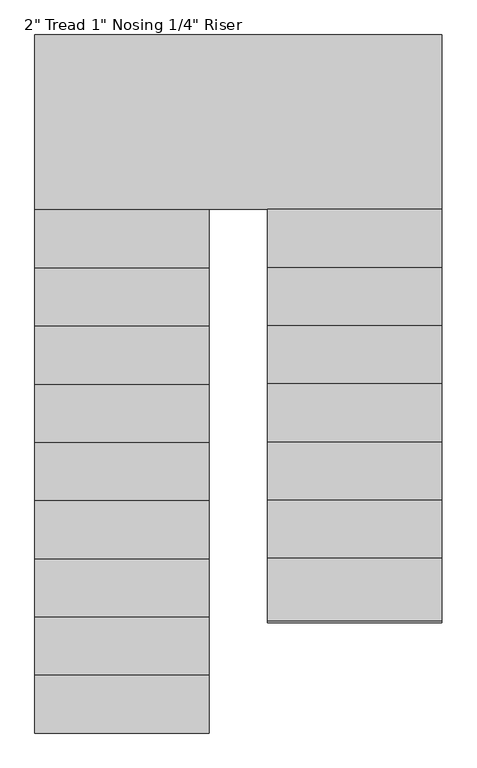
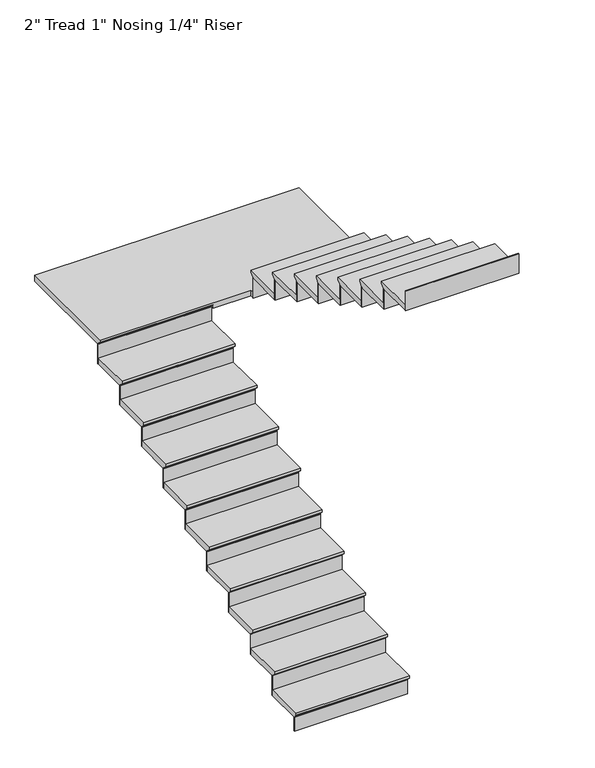
"""IFC4 building model written with IfcOpenShell, lengths in millimetres: stair flight geometry."""

from ifc_helpers import new_model, si_unit, origin, place, context, project, spatial, faceted_brep, source, transform, mapped, element, save


def stair_flight_5b78524c(model_context):
    return source(origin(), model_context, "Body", "Brep", [
        faceted_brep([(-77.7175798, -12221.8061634, 455.0833333), (-77.7175798, -12221.8061634, 474.1333333), (-992.1175798, -12221.8061634, 474.1333333), (-992.1175798, -12221.8061634, 455.0833333), (-77.7175798, -12196.4061634, 429.6833333), (-992.1175798, -12196.4061634, 429.6833333), (-77.7175798, -11891.6061634, 474.1333333), (-992.1175798, -11891.6061634, 474.1333333), (-992.1175798, -12196.4061634, 423.3333333), (-992.1175798, -11891.6061634, 423.3333333), (-77.7175798, -11891.6061634, 423.3333333), (-77.7175798, -12196.4061634, 423.3333333)], [[[0, 1, 2, 3]], [[4, 0, 3, 5]], [[2, 1, 6, 7]], [[8, 9, 10, 11]], [[2, 7, 9, 8, 5, 3]], [[8, 11, 4, 5]], [[6, 1, 0, 4, 11, 10]], [[7, 6, 10, 9]]]),
        faceted_brep([(-77.7175798, -12196.4061634, 423.3333333), (-77.7175798, -12196.4061634, 304.8), (-77.7175798, -12190.0561634, 304.8), (-77.7175798, -12190.0561634, 423.3333333), (-992.1175798, -12196.4061634, 423.3333333), (-992.1175798, -12190.0561634, 423.3333333), (-992.1175798, -12190.0561634, 304.8), (-992.1175798, -12196.4061634, 304.8)], [[[0, 1, 2, 3]], [[4, 5, 6, 7]], [[1, 0, 4, 7]], [[2, 1, 7, 6]], [[3, 2, 6, 5]], [[0, 3, 5, 4]]]),
        faceted_brep([(-77.7175798, -11891.6061634, 592.6666667), (-77.7175798, -11891.6061634, 423.3333333), (-77.7175798, -11885.2561634, 423.3333333), (-77.7175798, -11885.2561634, 592.6666667), (-992.1175798, -11891.6061634, 592.6666667), (-992.1175798, -11885.2561634, 592.6666667), (-992.1175798, -11885.2561634, 423.3333333), (-992.1175798, -11891.6061634, 423.3333333)], [[[0, 1, 2, 3]], [[4, 5, 6, 7]], [[1, 0, 4, 7]], [[2, 1, 7, 6]], [[3, 2, 6, 5]], [[0, 3, 5, 4]]]),
        faceted_brep([(-992.1175798, -11917.0061634, 643.4666667), (-77.7175798, -11917.0061634, 643.4666667), (-77.7175798, -11586.8061634, 643.4666667), (-992.1175798, -11586.8061634, 643.4666667), (-992.1175798, -11891.6061634, 592.6666667), (-992.1175798, -11586.8061634, 592.6666667), (-77.7175798, -11586.8061634, 592.6666667), (-77.7175798, -11891.6061634, 592.6666667), (-992.1175798, -11891.6061634, 599.0166667), (-992.1175798, -11917.0061634, 624.4166667), (-77.7175798, -11891.6061634, 599.0166667), (-77.7175798, -11917.0061634, 624.4166667)], [[[0, 1, 2, 3]], [[4, 5, 6, 7]], [[0, 3, 5, 4, 8, 9]], [[4, 7, 10, 8]], [[2, 1, 11, 10, 7, 6]], [[3, 2, 6, 5]], [[11, 1, 0, 9]], [[10, 11, 9, 8]]]),
        faceted_brep([(-77.7175798, -11586.8061634, 762.0), (-77.7175798, -11586.8061634, 592.6666667), (-77.7175798, -11580.4561634, 592.6666667), (-77.7175798, -11580.4561634, 762.0), (-992.1175798, -11586.8061634, 762.0), (-992.1175798, -11580.4561634, 762.0), (-992.1175798, -11580.4561634, 592.6666667), (-992.1175798, -11586.8061634, 592.6666667)], [[[0, 1, 2, 3]], [[4, 5, 6, 7]], [[1, 0, 4, 7]], [[2, 1, 7, 6]], [[3, 2, 6, 5]], [[0, 3, 5, 4]]]),
        faceted_brep([(-992.1175798, -11612.2061634, 812.8), (-77.7175798, -11612.2061634, 812.8), (-77.7175798, -11282.0061634, 812.8), (-992.1175798, -11282.0061634, 812.8), (-992.1175798, -11586.8061634, 762.0), (-992.1175798, -11282.0061634, 762.0), (-77.7175798, -11282.0061634, 762.0), (-77.7175798, -11586.8061634, 762.0), (-992.1175798, -11586.8061634, 768.35), (-992.1175798, -11612.2061634, 793.75), (-77.7175798, -11586.8061634, 768.35), (-77.7175798, -11612.2061634, 793.75)], [[[0, 1, 2, 3]], [[4, 5, 6, 7]], [[0, 3, 5, 4, 8, 9]], [[4, 7, 10, 8]], [[2, 1, 11, 10, 7, 6]], [[3, 2, 6, 5]], [[11, 1, 0, 9]], [[10, 11, 9, 8]]]),
        faceted_brep([(-77.7175798, -11282.0061634, 931.3333333), (-77.7175798, -11282.0061634, 762.0), (-77.7175798, -11275.6561634, 762.0), (-77.7175798, -11275.6561634, 931.3333333), (-992.1175798, -11282.0061634, 931.3333333), (-992.1175798, -11275.6561634, 931.3333333), (-992.1175798, -11275.6561634, 762.0), (-992.1175798, -11282.0061634, 762.0)], [[[0, 1, 2, 3]], [[4, 5, 6, 7]], [[1, 0, 4, 7]], [[2, 1, 7, 6]], [[3, 2, 6, 5]], [[0, 3, 5, 4]]]),
        faceted_brep([(-992.1175798, -11307.4061634, 982.1333333), (-77.7175798, -11307.4061634, 982.1333333), (-77.7175798, -10977.2061634, 982.1333333), (-992.1175798, -10977.2061634, 982.1333333), (-992.1175798, -11282.0061634, 931.3333333), (-992.1175798, -10977.2061634, 931.3333333), (-77.7175798, -10977.2061634, 931.3333333), (-77.7175798, -11282.0061634, 931.3333333), (-992.1175798, -11282.0061634, 937.6833333), (-992.1175798, -11307.4061634, 963.0833333), (-77.7175798, -11282.0061634, 937.6833333), (-77.7175798, -11307.4061634, 963.0833333)], [[[0, 1, 2, 3]], [[4, 5, 6, 7]], [[0, 3, 5, 4, 8, 9]], [[4, 7, 10, 8]], [[2, 1, 11, 10, 7, 6]], [[3, 2, 6, 5]], [[11, 1, 0, 9]], [[10, 11, 9, 8]]]),
        faceted_brep([(-77.7175798, -10977.2061634, 1100.6666667), (-77.7175798, -10977.2061634, 931.3333333), (-77.7175798, -10970.8561634, 931.3333333), (-77.7175798, -10970.8561634, 1100.6666667), (-992.1175798, -10977.2061634, 1100.6666667), (-992.1175798, -10970.8561634, 1100.6666667), (-992.1175798, -10970.8561634, 931.3333333), (-992.1175798, -10977.2061634, 931.3333333)], [[[0, 1, 2, 3]], [[4, 5, 6, 7]], [[1, 0, 4, 7]], [[2, 1, 7, 6]], [[3, 2, 6, 5]], [[0, 3, 5, 4]]]),
        faceted_brep([(-992.1175798, -11002.6061634, 1151.4666667), (-77.7175798, -11002.6061634, 1151.4666667), (-77.7175798, -10672.4061634, 1151.4666667), (-992.1175798, -10672.4061634, 1151.4666667), (-992.1175798, -10977.2061634, 1100.6666667), (-992.1175798, -10672.4061634, 1100.6666667), (-77.7175798, -10672.4061634, 1100.6666667), (-77.7175798, -10977.2061634, 1100.6666667), (-992.1175798, -10977.2061634, 1107.0166667), (-992.1175798, -11002.6061634, 1132.4166667), (-77.7175798, -10977.2061634, 1107.0166667), (-77.7175798, -11002.6061634, 1132.4166667)], [[[0, 1, 2, 3]], [[4, 5, 6, 7]], [[0, 3, 5, 4, 8, 9]], [[4, 7, 10, 8]], [[2, 1, 11, 10, 7, 6]], [[3, 2, 6, 5]], [[11, 1, 0, 9]], [[10, 11, 9, 8]]]),
        faceted_brep([(-77.7175798, -10672.4061634, 1270.0), (-77.7175798, -10672.4061634, 1100.6666667), (-77.7175798, -10666.0561634, 1100.6666667), (-77.7175798, -10666.0561634, 1270.0), (-992.1175798, -10672.4061634, 1270.0), (-992.1175798, -10666.0561634, 1270.0), (-992.1175798, -10666.0561634, 1100.6666667), (-992.1175798, -10672.4061634, 1100.6666667)], [[[0, 1, 2, 3]], [[4, 5, 6, 7]], [[1, 0, 4, 7]], [[2, 1, 7, 6]], [[3, 2, 6, 5]], [[0, 3, 5, 4]]]),
        faceted_brep([(-992.1175798, -10697.8061634, 1320.8), (-77.7175798, -10697.8061634, 1320.8), (-77.7175798, -10367.6061634, 1320.8), (-992.1175798, -10367.6061634, 1320.8), (-992.1175798, -10672.4061634, 1270.0), (-992.1175798, -10367.6061634, 1270.0), (-77.7175798, -10367.6061634, 1270.0), (-77.7175798, -10672.4061634, 1270.0), (-992.1175798, -10672.4061634, 1276.35), (-992.1175798, -10697.8061634, 1301.75), (-77.7175798, -10672.4061634, 1276.35), (-77.7175798, -10697.8061634, 1301.75)], [[[0, 1, 2, 3]], [[4, 5, 6, 7]], [[0, 3, 5, 4, 8, 9]], [[4, 7, 10, 8]], [[2, 1, 11, 10, 7, 6]], [[3, 2, 6, 5]], [[11, 1, 0, 9]], [[10, 11, 9, 8]]]),
        faceted_brep([(-77.7175798, -10367.6061634, 1439.3333333), (-77.7175798, -10367.6061634, 1270.0), (-77.7175798, -10361.2561634, 1270.0), (-77.7175798, -10361.2561634, 1439.3333333), (-992.1175798, -10367.6061634, 1439.3333333), (-992.1175798, -10361.2561634, 1439.3333333), (-992.1175798, -10361.2561634, 1270.0), (-992.1175798, -10367.6061634, 1270.0)], [[[0, 1, 2, 3]], [[4, 5, 6, 7]], [[1, 0, 4, 7]], [[2, 1, 7, 6]], [[3, 2, 6, 5]], [[0, 3, 5, 4]]]),
        faceted_brep([(-992.1175798, -10393.0061634, 1490.1333333), (-77.7175798, -10393.0061634, 1490.1333333), (-77.7175798, -10062.8061634, 1490.1333333), (-992.1175798, -10062.8061634, 1490.1333333), (-992.1175798, -10367.6061634, 1439.3333333), (-992.1175798, -10062.8061634, 1439.3333333), (-77.7175798, -10062.8061634, 1439.3333333), (-77.7175798, -10367.6061634, 1439.3333333), (-992.1175798, -10367.6061634, 1445.6833333), (-992.1175798, -10393.0061634, 1471.0833333), (-77.7175798, -10367.6061634, 1445.6833333), (-77.7175798, -10393.0061634, 1471.0833333)], [[[0, 1, 2, 3]], [[4, 5, 6, 7]], [[0, 3, 5, 4, 8, 9]], [[4, 7, 10, 8]], [[2, 1, 11, 10, 7, 6]], [[3, 2, 6, 5]], [[11, 1, 0, 9]], [[10, 11, 9, 8]]]),
        faceted_brep([(-77.7175798, -10062.8061634, 1608.6666667), (-77.7175798, -10062.8061634, 1439.3333333), (-77.7175798, -10056.4561634, 1439.3333333), (-77.7175798, -10056.4561634, 1608.6666667), (-992.1175798, -10062.8061634, 1608.6666667), (-992.1175798, -10056.4561634, 1608.6666667), (-992.1175798, -10056.4561634, 1439.3333333), (-992.1175798, -10062.8061634, 1439.3333333)], [[[0, 1, 2, 3]], [[4, 5, 6, 7]], [[1, 0, 4, 7]], [[2, 1, 7, 6]], [[3, 2, 6, 5]], [[0, 3, 5, 4]]]),
        faceted_brep([(-992.1175798, -10088.2061634, 1659.4666667), (-77.7175798, -10088.2061634, 1659.4666667), (-77.7175798, -9758.0061634, 1659.4666667), (-992.1175798, -9758.0061634, 1659.4666667), (-992.1175798, -10062.8061634, 1608.6666667), (-992.1175798, -9758.0061634, 1608.6666667), (-77.7175798, -9758.0061634, 1608.6666667), (-77.7175798, -10062.8061634, 1608.6666667), (-992.1175798, -10062.8061634, 1615.0166667), (-992.1175798, -10088.2061634, 1640.4166667), (-77.7175798, -10062.8061634, 1615.0166667), (-77.7175798, -10088.2061634, 1640.4166667)], [[[0, 1, 2, 3]], [[4, 5, 6, 7]], [[0, 3, 5, 4, 8, 9]], [[4, 7, 10, 8]], [[2, 1, 11, 10, 7, 6]], [[3, 2, 6, 5]], [[11, 1, 0, 9]], [[10, 11, 9, 8]]]),
        faceted_brep([(-77.7175798, -9758.0061634, 1778.0), (-77.7175798, -9758.0061634, 1608.6666667), (-77.7175798, -9751.6561634, 1608.6666667), (-77.7175798, -9751.6561634, 1778.0), (-992.1175798, -9758.0061634, 1778.0), (-992.1175798, -9751.6561634, 1778.0), (-992.1175798, -9751.6561634, 1608.6666667), (-992.1175798, -9758.0061634, 1608.6666667)], [[[0, 1, 2, 3]], [[4, 5, 6, 7]], [[1, 0, 4, 7]], [[2, 1, 7, 6]], [[3, 2, 6, 5]], [[0, 3, 5, 4]]]),
        faceted_brep([(-992.1175798, -9783.4061634, 1828.8), (-77.7175798, -9783.4061634, 1828.8), (-77.7175798, -9453.2061634, 1828.8), (-992.1175798, -9453.2061634, 1828.8), (-992.1175798, -9758.0061634, 1778.0), (-992.1175798, -9453.2061634, 1778.0), (-77.7175798, -9453.2061634, 1778.0), (-77.7175798, -9758.0061634, 1778.0), (-992.1175798, -9758.0061634, 1784.35), (-992.1175798, -9783.4061634, 1809.75), (-77.7175798, -9758.0061634, 1784.35), (-77.7175798, -9783.4061634, 1809.75)], [[[0, 1, 2, 3]], [[4, 5, 6, 7]], [[0, 3, 5, 4, 8, 9]], [[4, 7, 10, 8]], [[2, 1, 11, 10, 7, 6]], [[3, 2, 6, 5]], [[11, 1, 0, 9]], [[10, 11, 9, 8]]]),
        faceted_brep([(-77.7175798, -9453.2061634, 1947.3333333), (-77.7175798, -9453.2061634, 1778.0), (-77.7175798, -9446.8561634, 1778.0), (-77.7175798, -9446.8561634, 1947.3333333), (-992.1175798, -9453.2061634, 1947.3333333), (-992.1175798, -9446.8561634, 1947.3333333), (-992.1175798, -9446.8561634, 1778.0), (-992.1175798, -9453.2061634, 1778.0)], [[[0, 1, 2, 3]], [[4, 5, 6, 7]], [[1, 0, 4, 7]], [[2, 1, 7, 6]], [[3, 2, 6, 5]], [[0, 3, 5, 4]]]),
        faceted_brep([(1141.4824202, -9504.0061634, 1998.1333333), (1141.4824202, -8564.2061634, 1998.1333333), (-992.1175798, -8564.2061634, 1998.1333333), (-992.1175798, -9478.6061634, 1998.1333333), (227.0824202, -9478.6061634, 1998.1333333), (227.0824202, -9504.0061634, 1998.1333333), (1141.4824202, -8564.2061634, 1947.3333333), (1141.4824202, -9504.0061634, 1947.3333333), (227.0824202, -9504.0061634, 1947.3333333), (227.0824202, -9478.6061634, 1947.3333333), (-77.7175798, -9478.6061634, 1947.3333333), (-77.7175798, -9453.2061634, 1947.3333333), (-992.1175798, -9453.2061634, 1947.3333333), (-992.1175798, -8564.2061634, 1947.3333333), (-992.1175798, -9453.2061634, 1953.6833333), (-992.1175798, -9478.6061634, 1979.0833333), (-77.7175798, -9453.2061634, 1953.6833333), (-77.7175798, -9478.6061634, 1979.0833333)], [[[0, 1, 2, 3, 4, 5]], [[6, 7, 8, 9, 10, 11, 12, 13]], [[1, 0, 7, 6]], [[2, 1, 6, 13]], [[3, 2, 13, 12, 14, 15]], [[12, 11, 16, 14]], [[11, 10, 17, 16]], [[4, 3, 15, 17, 10, 9]], [[5, 4, 9, 8]], [[0, 5, 8, 7]], [[15, 14, 16, 17]]]),
        faceted_brep([(227.0824202, -9504.0061634, 2116.6666667), (227.0824202, -9504.0061634, 1947.3333333), (227.0824202, -9510.3561634, 1947.3333333), (227.0824202, -9510.3561634, 2116.6666667), (1141.4824202, -9504.0061634, 2116.6666667), (1141.4824202, -9510.3561634, 2116.6666667), (1141.4824202, -9510.3561634, 1947.3333333), (1141.4824202, -9504.0061634, 1947.3333333)], [[[0, 1, 2, 3]], [[4, 5, 6, 7]], [[1, 0, 4, 7]], [[2, 1, 7, 6]], [[3, 2, 6, 5]], [[0, 3, 5, 4]]]),
        faceted_brep([(1141.4824202, -9478.6061634, 2167.4666667), (227.0824202, -9478.6061634, 2167.4666667), (227.0824202, -9808.8061634, 2167.4666667), (1141.4824202, -9808.8061634, 2167.4666667), (1141.4824202, -9504.0061634, 2116.6666667), (1141.4824202, -9808.8061634, 2116.6666667), (227.0824202, -9808.8061634, 2116.6666667), (227.0824202, -9504.0061634, 2116.6666667), (1141.4824202, -9504.0061634, 2123.0166667), (1141.4824202, -9478.6061634, 2148.4166667), (227.0824202, -9504.0061634, 2123.0166667), (227.0824202, -9478.6061634, 2148.4166667)], [[[0, 1, 2, 3]], [[4, 5, 6, 7]], [[0, 3, 5, 4, 8, 9]], [[4, 7, 10, 8]], [[2, 1, 11, 10, 7, 6]], [[3, 2, 6, 5]], [[11, 1, 0, 9]], [[10, 11, 9, 8]]]),
        faceted_brep([(227.0824202, -9808.8061634, 2286.0), (227.0824202, -9808.8061634, 2116.6666667), (227.0824202, -9815.1561634, 2116.6666667), (227.0824202, -9815.1561634, 2286.0), (1141.4824202, -9808.8061634, 2286.0), (1141.4824202, -9815.1561634, 2286.0), (1141.4824202, -9815.1561634, 2116.6666667), (1141.4824202, -9808.8061634, 2116.6666667)], [[[0, 1, 2, 3]], [[4, 5, 6, 7]], [[1, 0, 4, 7]], [[2, 1, 7, 6]], [[3, 2, 6, 5]], [[0, 3, 5, 4]]]),
        faceted_brep([(1141.4824202, -9783.4061634, 2336.8), (227.0824202, -9783.4061634, 2336.8), (227.0824202, -10113.6061634, 2336.8), (1141.4824202, -10113.6061634, 2336.8), (1141.4824202, -9808.8061634, 2286.0), (1141.4824202, -10113.6061634, 2286.0), (227.0824202, -10113.6061634, 2286.0), (227.0824202, -9808.8061634, 2286.0), (1141.4824202, -9808.8061634, 2292.35), (1141.4824202, -9783.4061634, 2317.75), (227.0824202, -9808.8061634, 2292.35), (227.0824202, -9783.4061634, 2317.75)], [[[0, 1, 2, 3]], [[4, 5, 6, 7]], [[0, 3, 5, 4, 8, 9]], [[4, 7, 10, 8]], [[2, 1, 11, 10, 7, 6]], [[3, 2, 6, 5]], [[11, 1, 0, 9]], [[10, 11, 9, 8]]]),
        faceted_brep([(227.0824202, -10113.6061634, 2455.3333333), (227.0824202, -10113.6061634, 2286.0), (227.0824202, -10119.9561634, 2286.0), (227.0824202, -10119.9561634, 2455.3333333), (1141.4824202, -10113.6061634, 2455.3333333), (1141.4824202, -10119.9561634, 2455.3333333), (1141.4824202, -10119.9561634, 2286.0), (1141.4824202, -10113.6061634, 2286.0)], [[[0, 1, 2, 3]], [[4, 5, 6, 7]], [[1, 0, 4, 7]], [[2, 1, 7, 6]], [[3, 2, 6, 5]], [[0, 3, 5, 4]]]),
        faceted_brep([(1141.4824202, -10088.2061634, 2506.1333333), (227.0824202, -10088.2061634, 2506.1333333), (227.0824202, -10418.4061634, 2506.1333333), (1141.4824202, -10418.4061634, 2506.1333333), (1141.4824202, -10113.6061634, 2455.3333333), (1141.4824202, -10418.4061634, 2455.3333333), (227.0824202, -10418.4061634, 2455.3333333), (227.0824202, -10113.6061634, 2455.3333333), (1141.4824202, -10113.6061634, 2461.6833333), (1141.4824202, -10088.2061634, 2487.0833333), (227.0824202, -10113.6061634, 2461.6833333), (227.0824202, -10088.2061634, 2487.0833333)], [[[0, 1, 2, 3]], [[4, 5, 6, 7]], [[0, 3, 5, 4, 8, 9]], [[4, 7, 10, 8]], [[2, 1, 11, 10, 7, 6]], [[3, 2, 6, 5]], [[11, 1, 0, 9]], [[10, 11, 9, 8]]]),
        faceted_brep([(227.0824202, -10418.4061634, 2624.6666667), (227.0824202, -10418.4061634, 2455.3333333), (227.0824202, -10424.7561634, 2455.3333333), (227.0824202, -10424.7561634, 2624.6666667), (1141.4824202, -10418.4061634, 2624.6666667), (1141.4824202, -10424.7561634, 2624.6666667), (1141.4824202, -10424.7561634, 2455.3333333), (1141.4824202, -10418.4061634, 2455.3333333)], [[[0, 1, 2, 3]], [[4, 5, 6, 7]], [[1, 0, 4, 7]], [[2, 1, 7, 6]], [[3, 2, 6, 5]], [[0, 3, 5, 4]]]),
        faceted_brep([(1141.4824202, -10393.0061634, 2675.4666667), (227.0824202, -10393.0061634, 2675.4666667), (227.0824202, -10723.2061634, 2675.4666667), (1141.4824202, -10723.2061634, 2675.4666667), (1141.4824202, -10418.4061634, 2624.6666667), (1141.4824202, -10723.2061634, 2624.6666667), (227.0824202, -10723.2061634, 2624.6666667), (227.0824202, -10418.4061634, 2624.6666667), (1141.4824202, -10418.4061634, 2631.0166667), (1141.4824202, -10393.0061634, 2656.4166667), (227.0824202, -10418.4061634, 2631.0166667), (227.0824202, -10393.0061634, 2656.4166667)], [[[0, 1, 2, 3]], [[4, 5, 6, 7]], [[0, 3, 5, 4, 8, 9]], [[4, 7, 10, 8]], [[2, 1, 11, 10, 7, 6]], [[3, 2, 6, 5]], [[11, 1, 0, 9]], [[10, 11, 9, 8]]]),
        faceted_brep([(227.0824202, -10723.2061634, 2794.0), (227.0824202, -10723.2061634, 2624.6666667), (227.0824202, -10729.5561634, 2624.6666667), (227.0824202, -10729.5561634, 2794.0), (1141.4824202, -10723.2061634, 2794.0), (1141.4824202, -10729.5561634, 2794.0), (1141.4824202, -10729.5561634, 2624.6666667), (1141.4824202, -10723.2061634, 2624.6666667)], [[[0, 1, 2, 3]], [[4, 5, 6, 7]], [[1, 0, 4, 7]], [[2, 1, 7, 6]], [[3, 2, 6, 5]], [[0, 3, 5, 4]]]),
        faceted_brep([(1141.4824202, -10697.8061634, 2844.8), (227.0824202, -10697.8061634, 2844.8), (227.0824202, -11028.0061634, 2844.8), (1141.4824202, -11028.0061634, 2844.8), (1141.4824202, -10723.2061634, 2794.0), (1141.4824202, -11028.0061634, 2794.0), (227.0824202, -11028.0061634, 2794.0), (227.0824202, -10723.2061634, 2794.0), (1141.4824202, -10723.2061634, 2800.35), (1141.4824202, -10697.8061634, 2825.75), (227.0824202, -10723.2061634, 2800.35), (227.0824202, -10697.8061634, 2825.75)], [[[0, 1, 2, 3]], [[4, 5, 6, 7]], [[0, 3, 5, 4, 8, 9]], [[4, 7, 10, 8]], [[2, 1, 11, 10, 7, 6]], [[3, 2, 6, 5]], [[11, 1, 0, 9]], [[10, 11, 9, 8]]]),
        faceted_brep([(227.0824202, -11028.0061634, 2963.3333333), (227.0824202, -11028.0061634, 2794.0), (227.0824202, -11034.3561634, 2794.0), (227.0824202, -11034.3561634, 2963.3333333), (1141.4824202, -11028.0061634, 2963.3333333), (1141.4824202, -11034.3561634, 2963.3333333), (1141.4824202, -11034.3561634, 2794.0), (1141.4824202, -11028.0061634, 2794.0)], [[[0, 1, 2, 3]], [[4, 5, 6, 7]], [[1, 0, 4, 7]], [[2, 1, 7, 6]], [[3, 2, 6, 5]], [[0, 3, 5, 4]]]),
        faceted_brep([(1141.4824202, -11002.6061634, 3014.1333333), (227.0824202, -11002.6061634, 3014.1333333), (227.0824202, -11332.8061634, 3014.1333333), (1141.4824202, -11332.8061634, 3014.1333333), (1141.4824202, -11028.0061634, 2963.3333333), (1141.4824202, -11332.8061634, 2963.3333333), (227.0824202, -11332.8061634, 2963.3333333), (227.0824202, -11028.0061634, 2963.3333333), (1141.4824202, -11028.0061634, 2969.6833333), (1141.4824202, -11002.6061634, 2995.0833333), (227.0824202, -11028.0061634, 2969.6833333), (227.0824202, -11002.6061634, 2995.0833333)], [[[0, 1, 2, 3]], [[4, 5, 6, 7]], [[0, 3, 5, 4, 8, 9]], [[4, 7, 10, 8]], [[2, 1, 11, 10, 7, 6]], [[3, 2, 6, 5]], [[11, 1, 0, 9]], [[10, 11, 9, 8]]]),
        faceted_brep([(227.0824202, -11332.8061634, 3132.6666667), (227.0824202, -11332.8061634, 2963.3333333), (227.0824202, -11339.1561634, 2963.3333333), (227.0824202, -11339.1561634, 3132.6666667), (1141.4824202, -11332.8061634, 3132.6666667), (1141.4824202, -11339.1561634, 3132.6666667), (1141.4824202, -11339.1561634, 2963.3333333), (1141.4824202, -11332.8061634, 2963.3333333)], [[[0, 1, 2, 3]], [[4, 5, 6, 7]], [[1, 0, 4, 7]], [[2, 1, 7, 6]], [[3, 2, 6, 5]], [[0, 3, 5, 4]]]),
        faceted_brep([(227.0824202, -11637.6061634, 3302.0), (227.0824202, -11637.6061634, 3132.6666667), (227.0824202, -11643.9561634, 3132.6666667), (227.0824202, -11643.9561634, 3302.0), (1141.4824202, -11637.6061634, 3302.0), (1141.4824202, -11643.9561634, 3302.0), (1141.4824202, -11643.9561634, 3132.6666667), (1141.4824202, -11637.6061634, 3132.6666667)], [[[0, 1, 2, 3]], [[4, 5, 6, 7]], [[1, 0, 4, 7]], [[2, 1, 7, 6]], [[3, 2, 6, 5]], [[0, 3, 5, 4]]]),
        faceted_brep([(1141.4824202, -11307.4061634, 3183.4666667), (227.0824202, -11307.4061634, 3183.4666667), (227.0824202, -11637.6061634, 3183.4666667), (1141.4824202, -11637.6061634, 3183.4666667), (1141.4824202, -11332.8061634, 3132.6666667), (1141.4824202, -11637.6061634, 3132.6666667), (227.0824202, -11637.6061634, 3132.6666667), (227.0824202, -11332.8061634, 3132.6666667), (1141.4824202, -11332.8061634, 3139.0166667), (1141.4824202, -11307.4061634, 3164.4166667), (227.0824202, -11332.8061634, 3139.0166667), (227.0824202, -11307.4061634, 3164.4166667)], [[[0, 1, 2, 3]], [[4, 5, 6, 7]], [[0, 3, 5, 4, 8, 9]], [[4, 7, 10, 8]], [[2, 1, 11, 10, 7, 6]], [[3, 2, 6, 5]], [[11, 1, 0, 9]], [[10, 11, 9, 8]]]),
    ])


if __name__ == "__main__":
    model = new_model("IFC4")
    model_context = context("Model", 3, world=origin())
    ifc_project = project(units=[si_unit("LENGTHUNIT", "METRE", prefix="MILLI")], contexts=[model_context])
    site = spatial("IfcSite", under=ifc_project)
    building = spatial("IfcBuilding", under=site)
    placement = place(None, origin())
    stair_flight_shape = stair_flight_5b78524c(model_context)
    element("IfcStairFlight", 1, ObjectType="2\" Tread 1\" Nosing 1/4\" Riser", at=placement, inside=building, context=model_context, shape_type="MappedRepresentation", body=[
        mapped(stair_flight_shape, transform((0.0, 0.0, 0.0), x_axis=(1.0, 0.0, 0.0), y_axis=(0.0, 1.0, 0.0), z_axis=(0.0, 0.0, 1.0))),
    ])
    save(model, "model.ifc")

# Revit data of these elements
# Element 1 (IfcStairFlight, "2\" Tread 1\" Nosing 1/4\" Riser")
#   Materials on its faces: "FL_MARBLE WHITE"
# Materials
#   "FL_MARBLE WHITE": class "Generic", colour RGB 120 120 120, transparency 0, Cost = 0
